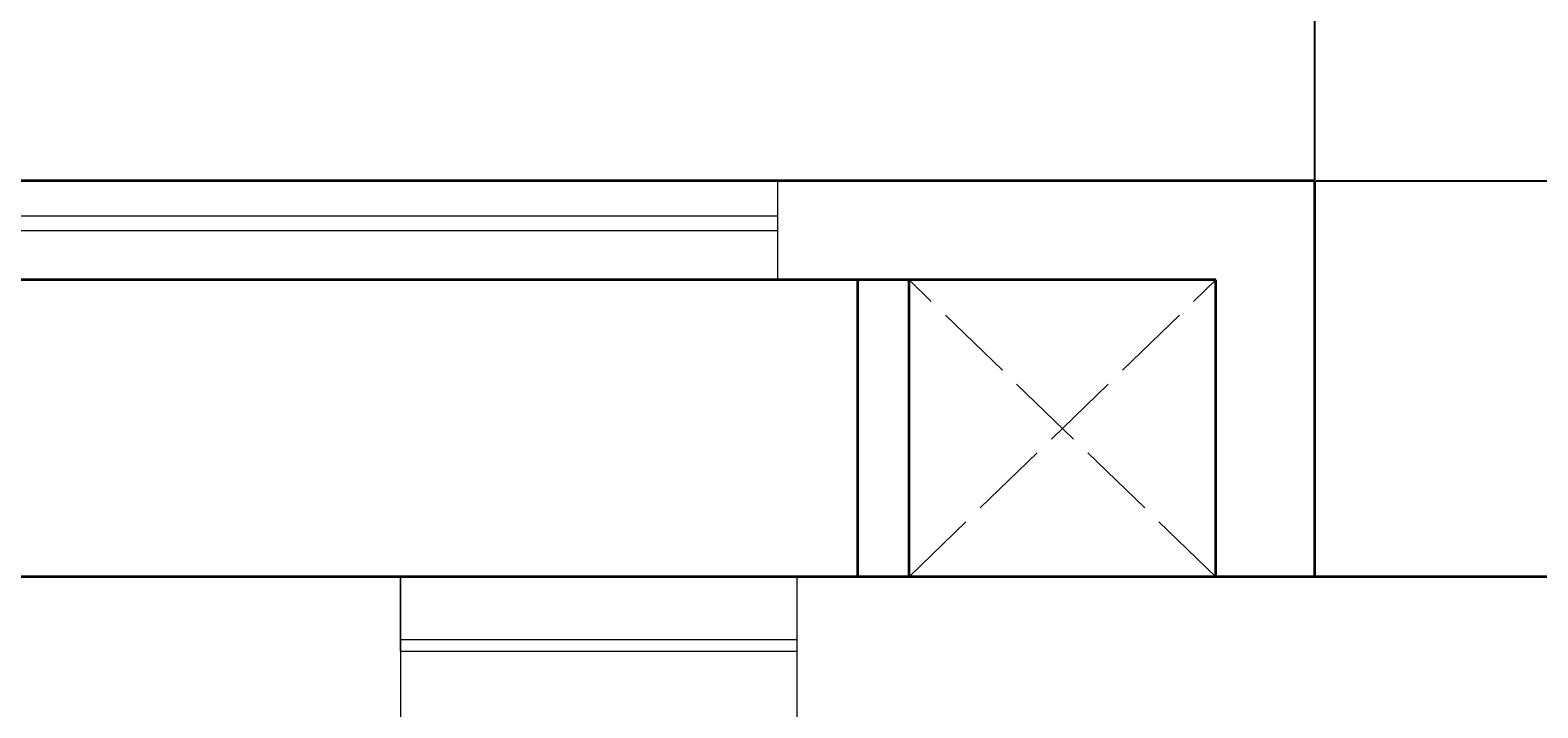
# Model space of a CAD drawing. Units: inches. Extents: x -61 to 1599, y -1316 to 257.
# Tile 176 of 204: x 1304 to 1395, y -620 to -579. Entities that reach past the tile are written whole.
import ezdxf

# ---------------------------------------------------------------- set-up
doc = ezdxf.new("R2010")
doc.units = ezdxf.units.IN
doc.header["$MEASUREMENT"] = 0
doc.linetypes.add('ACAD_ISO02W100', pattern=[15, 12, -3])
for name, color, linetype, lineweight in [('A-ANNO-DIMS', 2, 'Continuous', 18), ('A-FLOR-OPEN-HIDN', 8, 'ACAD_ISO02W100', 13), ('WALLS', 4, 'Continuous', 35), ('WINDOWS', 220, 'Continuous', 18)]:
    doc.layers.add(name, color=color, linetype=linetype, lineweight=lineweight)
doc.styles.get("Standard").update_dxf_attribs({"font": 'arial.ttf'})
doc.dimstyles.get("Standard").update_dxf_attribs({"dimtxt": 0.18, "dimasz": 0.18, "dimexe": 0.18, "dimexo": 0.0625, "dimgap": 0.09, "dimtad": 0, "dimtih": 1, "dimtoh": 1, "dimdec": 0, "dimzin": 0, "dimdsep": 46, "dimlunit": 3, "dimtxsty": 'Standard', "dimcen": 0.09, "dimadec": 0, "dimazin": 0, "dimtfac": 1, "dimtdec": 0, "dimtofl": 0, "dimtmove": 0, "dimatfit": 3, "dimfxl": 1, "dimtolj": 1, "dimtzin": 0, "dimarcsym": 0})

# ---------------------------------------------------------------- blocks, each defined once
blk = doc.blocks.new('WIN-24IN')
for p, q in [((0, 4.5), (0, 9)), ((0, 9), (0, 0)), ((24, 9), (24, 0)), ((0, 5.192), (24, 5.192)), ((0, 4.5), (24, 4.5))]:
    blk.add_line(p, q)
blk = doc.blocks.new('WIN-51IN')
for p, q in [((0, 0), (0, 6)), ((50.516, 0), (50.516, 6)), ((0, 3.885), (50.516, 3.885)), ((0, 3), (50.516, 3))]:
    blk.add_line(p, q)
blk = doc.blocks.new('*D708')
at = {"layer": 'A-ANNO-DIMS', "color": 0, "lineweight": -2, "transparency": 16777216}
for p, q in [((1267.481, -588.107), (1267.481, 257.457)), ((1267.661, 257.277), (1324.137, 257.277)), ((1381.523, 257.277), (1325.046, 257.277)), ((1381.703, -588.107), (1381.703, 257.457))]:
    blk.add_line(p, q, dxfattribs=at)
at = {"layer": 'A-ANNO-DIMS', "color": 0, "transparency": 16777216}
for points in [[(1267.661, 257.307), (1267.661, 257.247), (1267.481, 257.277)], [(1381.523, 257.307), (1381.523, 257.247), (1381.703, 257.277)]]:
    blk.add_solid(points, dxfattribs=at)
at = {"layer": 'DEFPOINTS', "color": 0, "transparency": 16777216}
for p in [(1381.703, 257.277), (1267.481, -588.169), (1381.703, -588.169)]:
    blk.add_point(p, dxfattribs=at)
at = {"layer": 'A-ANNO-DIMS', "color": 0, "transparency": 16777216, "insert": (1324.592, 257.277), "char_height": 0.18, "attachment_point": 5}
blk.add_mtext('\\A1;114.22', dxfattribs=at)
blk = doc.blocks.new('*D709')
at = {"layer": 'A-ANNO-DIMS', "color": 0, "lineweight": -2, "transparency": 16777216}
for p, q in [((1381.765, -588.169), (1598.483, -588.169)), ((1598.303, -588.349), (1598.303, -599.989)), ((1598.303, -611.989), (1598.303, -600.349)), ((1381.765, -612.169), (1598.483, -612.169))]:
    blk.add_line(p, q, dxfattribs=at)
at = {"layer": 'A-ANNO-DIMS', "color": 0, "transparency": 16777216}
for points in [[(1598.273, -588.349), (1598.333, -588.349), (1598.303, -588.169)], [(1598.273, -611.989), (1598.333, -611.989), (1598.303, -612.169)]]:
    blk.add_solid(points, dxfattribs=at)
at = {"layer": 'DEFPOINTS', "color": 0, "transparency": 16777216}
for p in [(1381.703, -588.169), (1381.703, -612.169), (1598.303, -612.169)]:
    blk.add_point(p, dxfattribs=at)
at = {"layer": 'A-ANNO-DIMS', "color": 0, "transparency": 16777216, "insert": (1598.303, -600.169), "char_height": 0.18, "attachment_point": 5}
blk.add_mtext('\\A1;24', dxfattribs=at)

msp = doc.modelspace()

# ---------------------------------------------------------------- linework, layer by layer
at = {"layer": 'A-FLOR-OPEN-HIDN', "ltscale": 0.4}
for p, q in [((1357.1186, -612.169), (1375.7028, -594.169)), ((1375.7028, -612.169), (1357.1186, -594.169))]:
    msp.add_line(p, q, dxfattribs=at)
at = {"layer": 'WALLS'}
for p, q in [((1381.7028, -588.169), (1267.4807, -588.169)), ((1381.7028, -612.169), (1381.7028, -588.169)), ((1375.7028, -594.169), (1273.4807, -594.169)), ((1354.0257, -612.169), (1354.0257, -594.169)), ((1357.1186, -612.169), (1357.1186, -594.169)), ((1375.7028, -612.169), (1375.7028, -594.169)), ((1522.7028, -612.169), (992.7028, -612.169))]:
    msp.add_line(p, q, dxfattribs=at)

# ---------------------------------------------------------------- block references
at = {"layer": 'WINDOWS'}
for name, p in [('WIN-51IN', (1298.659, -594.1691)), ('WIN-24IN', (1326.3196, -621.1691))]:
    msp.add_blockref(name, p, dxfattribs=at)

# ---------------------------------------------------------------- dimensions: what is measured, and where the dimension line sits
at = {"layer": 'A-ANNO-DIMS'}
dim = msp.add_linear_dim(base=(1381.7028, 257.2771), p1=(1267.4807, -588.169), p2=(1381.7028, -588.169), dimstyle='Standard', override={"dimdec": 2, "dimlfac": 1, "dimrnd": 0, "dimzin": 0, "dimdsep": 46, "dimlunit": 2}, dxfattribs=at)
dim.commit()
dim.dimension.update_dxf_attribs({"geometry": '*D708', "text_midpoint": (1324.5917, 257.2771)})
dim = msp.add_linear_dim(base=(1598.3028, -612.169), p1=(1381.7028, -588.169), p2=(1381.7028, -612.169), angle=90, dimstyle='Standard', override={"dimdec": 0, "dimlfac": 1, "dimrnd": 0, "dimzin": 0, "dimdsep": 46, "dimlunit": 2}, dxfattribs=at)
dim.commit()
dim.dimension.update_dxf_attribs({"geometry": '*D709', "text_midpoint": (1598.3028, -600.169)})

doc.saveas('drawing.dxf')
